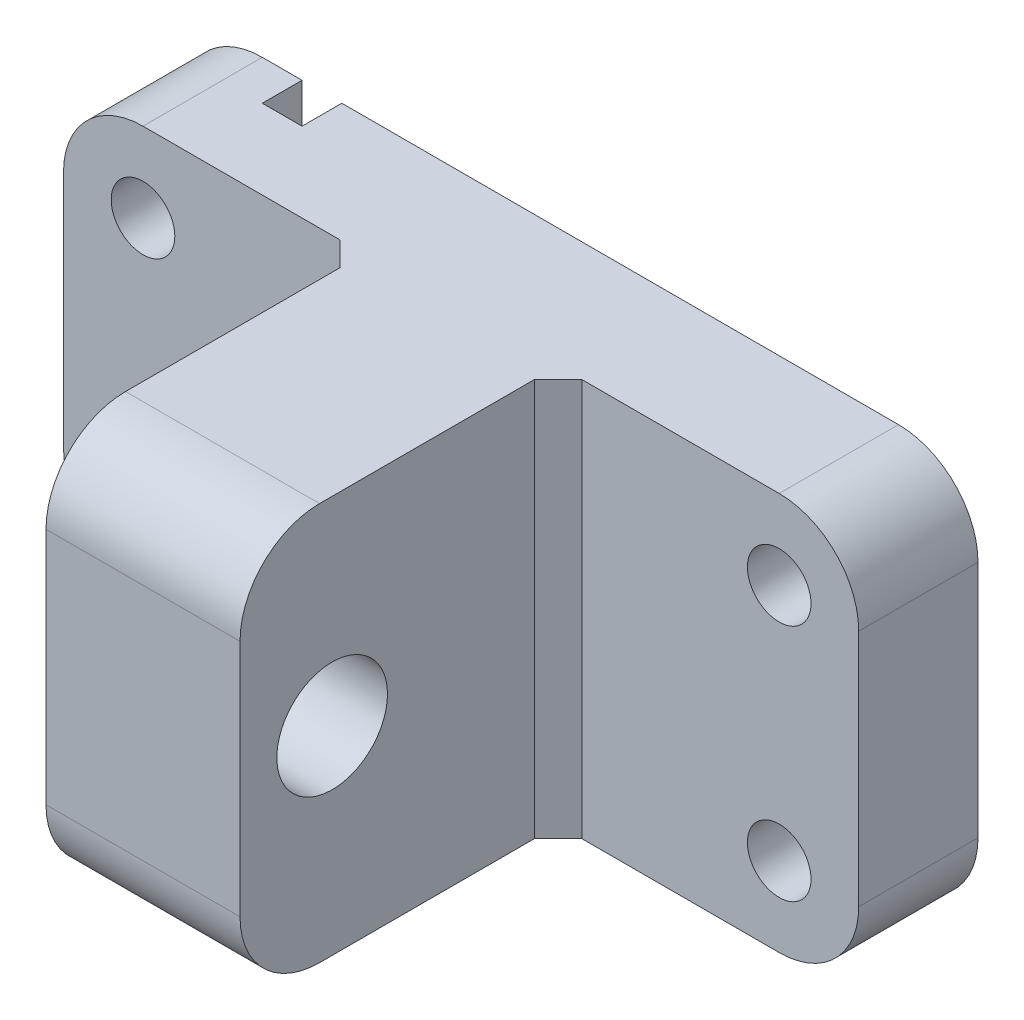
ISO-10303-21;
HEADER;
FILE_DESCRIPTION(('STEP AP214'),'2;1');
FILE_NAME('part.step','',(''),(''),'','','');
FILE_SCHEMA(('AUTOMOTIVE_DESIGN { 1 0 10303 214 1 1 1 1 }'));
ENDSEC;
DATA;
#1=APPLICATION_CONTEXT('core data for automotive mechanical design processes');
#2=APPLICATION_PROTOCOL_DEFINITION('international standard','automotive_design',2000,#1);
#3=PRODUCT_CONTEXT('',#1,'mechanical');
#4=PRODUCT('Part','Part','',(#3));
#5=PRODUCT_RELATED_PRODUCT_CATEGORY('part','',(#4));
#6=PRODUCT_DEFINITION_FORMATION('','',#4);
#7=PRODUCT_DEFINITION_CONTEXT('part definition',#1,'design');
#8=PRODUCT_DEFINITION('design','',#6,#7);
#9=PRODUCT_DEFINITION_SHAPE('','',#8);
#10=(LENGTH_UNIT() NAMED_UNIT(*) SI_UNIT(.MILLI.,.METRE.));
#11=(NAMED_UNIT(*) PLANE_ANGLE_UNIT() SI_UNIT($,.RADIAN.));
#12=(NAMED_UNIT(*) SI_UNIT($,.STERADIAN.) SOLID_ANGLE_UNIT());
#13=UNCERTAINTY_MEASURE_WITH_UNIT(LENGTH_MEASURE(1.E-05),#10,'distance_accuracy_value','');
#14=(GEOMETRIC_REPRESENTATION_CONTEXT(3) GLOBAL_UNCERTAINTY_ASSIGNED_CONTEXT((#13)) GLOBAL_UNIT_ASSIGNED_CONTEXT((#10,
#11,#12)) REPRESENTATION_CONTEXT('',''));
#15=CARTESIAN_POINT('',(0.,0.,0.));
#16=DIRECTION('',(0.,0.,1.));
#17=DIRECTION('',(1.,0.,0.));
#18=AXIS2_PLACEMENT_3D('',#15,#16,#17);
#19=CARTESIAN_POINT('',(90.,40.,0.));
#20=DIRECTION('',(0.,0.,1.));
#21=DIRECTION('',(1.,0.,0.));
#22=AXIS2_PLACEMENT_3D('',#19,#20,#21);
#23=PLANE('',#22);
#24=CARTESIAN_POINT('',(10.,40.,0.));
#25=DIRECTION('',(0.,0.,1.));
#26=DIRECTION('',(1.,0.,0.));
#27=AXIS2_PLACEMENT_3D('',#24,#25,#26);
#28=CIRCLE('',#27,4.);
#29=CARTESIAN_POINT('',(14.,40.,0.));
#30=VERTEX_POINT('',#29);
#31=EDGE_CURVE('E710',#30,#30,#28,.T.);
#32=ORIENTED_EDGE('',*,*,#31,.T.);
#33=EDGE_LOOP('',(#32));
#34=FACE_BOUND('',#33,.T.);
#35=CARTESIAN_POINT('',(10.,10.,0.));
#36=DIRECTION('',(0.,0.,1.));
#37=DIRECTION('',(1.,0.,0.));
#38=AXIS2_PLACEMENT_3D('',#35,#36,#37);
#39=CIRCLE('',#38,4.);
#40=CARTESIAN_POINT('',(14.,10.,0.));
#41=VERTEX_POINT('',#40);
#42=EDGE_CURVE('E712',#41,#41,#39,.T.);
#43=ORIENTED_EDGE('',*,*,#42,.T.);
#44=EDGE_LOOP('',(#43));
#45=FACE_BOUND('',#44,.T.);
#46=DIRECTION('',(-1.,0.,0.));
#47=VECTOR('',#46,1.);
#48=CARTESIAN_POINT('',(89.9999999999999,50.,0.));
#49=LINE('',#48,#47);
#50=CARTESIAN_POINT('',(15.,50.,0.));
#51=VERTEX_POINT('',#50);
#52=CARTESIAN_POINT('',(10.0000000000001,50.,0.));
#53=VERTEX_POINT('',#52);
#54=EDGE_CURVE('E287',#51,#53,#49,.T.);
#55=ORIENTED_EDGE('',*,*,#54,.F.);
#56=DIRECTION('',(0.,-1.,0.));
#57=VECTOR('',#56,1.);
#58=CARTESIAN_POINT('',(15.,50.,0.));
#59=LINE('',#58,#57);
#60=CARTESIAN_POINT('',(15.,0.,0.));
#61=VERTEX_POINT('',#60);
#62=EDGE_CURVE('E218',#51,#61,#59,.T.);
#63=ORIENTED_EDGE('',*,*,#62,.T.);
#64=DIRECTION('',(1.,0.,0.));
#65=VECTOR('',#64,1.);
#66=CARTESIAN_POINT('',(10.0000000000001,0.,0.));
#67=LINE('',#66,#65);
#68=CARTESIAN_POINT('',(10.0000000000001,0.,0.));
#69=VERTEX_POINT('',#68);
#70=EDGE_CURVE('E294',#69,#61,#67,.T.);
#71=ORIENTED_EDGE('',*,*,#70,.F.);
#72=CARTESIAN_POINT('',(10.,10.,0.));
#73=DIRECTION('',(0.,0.,1.));
#74=DIRECTION('',(-1.,0.,0.));
#75=AXIS2_PLACEMENT_3D('',#72,#73,#74);
#76=CIRCLE('',#75,10.);
#77=CARTESIAN_POINT('',(0.,10.,0.));
#78=VERTEX_POINT('',#77);
#79=EDGE_CURVE('E292',#78,#69,#76,.T.);
#80=ORIENTED_EDGE('',*,*,#79,.F.);
#81=DIRECTION('',(0.,-1.,0.));
#82=VECTOR('',#81,1.);
#83=CARTESIAN_POINT('',(0.,39.9999999999999,0.));
#84=LINE('',#83,#82);
#85=CARTESIAN_POINT('',(0.,39.9999999999999,0.));
#86=VERTEX_POINT('',#85);
#87=EDGE_CURVE('E288',#86,#78,#84,.T.);
#88=ORIENTED_EDGE('',*,*,#87,.F.);
#89=CARTESIAN_POINT('',(10.,40.,0.));
#90=DIRECTION('',(0.,0.,1.));
#91=DIRECTION('',(1.,0.,0.));
#92=AXIS2_PLACEMENT_3D('',#89,#90,#91);
#93=CIRCLE('',#92,10.);
#94=EDGE_CURVE('E290',#53,#86,#93,.T.);
#95=ORIENTED_EDGE('',*,*,#94,.F.);
#96=EDGE_LOOP('',(#55,#63,#71,#80,#88,#95));
#97=FACE_BOUND('',#96,.T.);
#98=ADVANCED_FACE('F50',(#34,#45,#97),#23,.F.);
#99=CARTESIAN_POINT('',(0.,10.,45.));
#100=DIRECTION('',(1.,0.,0.));
#101=DIRECTION('',(0.,0.,-1.));
#102=AXIS2_PLACEMENT_3D('',#99,#100,#101);
#103=CYLINDRICAL_SURFACE('',#102,10.);
#104=DIRECTION('',(1.,0.,0.));
#105=VECTOR('',#104,1.);
#106=CARTESIAN_POINT('',(0.,10.0000000000001,55.));
#107=LINE('',#106,#105);
#108=CARTESIAN_POINT('',(37.8,10.0000000000001,55.));
#109=VERTEX_POINT('',#108);
#110=CARTESIAN_POINT('',(62.2,9.99999999999993,55.));
#111=VERTEX_POINT('',#110);
#112=EDGE_CURVE('E267',#109,#111,#107,.T.);
#113=ORIENTED_EDGE('',*,*,#112,.F.);
#114=CARTESIAN_POINT('',(37.8,10.,45.));
#115=DIRECTION('',(-1.,0.,0.));
#116=DIRECTION('',(0.,0.,1.));
#117=AXIS2_PLACEMENT_3D('',#114,#115,#116);
#118=CIRCLE('',#117,10.);
#119=CARTESIAN_POINT('',(37.8,0.,45.0000000000001));
#120=VERTEX_POINT('',#119);
#121=EDGE_CURVE('E226',#120,#109,#118,.T.);
#122=ORIENTED_EDGE('',*,*,#121,.F.);
#123=DIRECTION('',(1.,0.,0.));
#124=VECTOR('',#123,1.);
#125=CARTESIAN_POINT('',(0.,0.,44.9999999999999));
#126=LINE('',#125,#124);
#127=CARTESIAN_POINT('',(62.2,0.,44.9999999999999));
#128=VERTEX_POINT('',#127);
#129=EDGE_CURVE('E265',#120,#128,#126,.T.);
#130=ORIENTED_EDGE('',*,*,#129,.T.);
#131=CARTESIAN_POINT('',(62.2,10.,45.));
#132=DIRECTION('',(1.,0.,0.));
#133=DIRECTION('',(0.,0.,-1.));
#134=AXIS2_PLACEMENT_3D('',#131,#132,#133);
#135=CIRCLE('',#134,10.);
#136=EDGE_CURVE('E252',#111,#128,#135,.T.);
#137=ORIENTED_EDGE('',*,*,#136,.F.);
#138=EDGE_LOOP('',(#113,#122,#130,#137));
#139=FACE_BOUND('',#138,.T.);
#140=ADVANCED_FACE('F348',(#139),#103,.T.);
#141=CARTESIAN_POINT('',(0.,39.9999999999999,55.));
#142=DIRECTION('',(0.,0.,1.));
#143=DIRECTION('',(1.,0.,0.));
#144=AXIS2_PLACEMENT_3D('',#141,#142,#143);
#145=PLANE('',#144);
#146=DIRECTION('',(1.,0.,0.));
#147=VECTOR('',#146,1.);
#148=CARTESIAN_POINT('',(0.,39.9999999999999,55.));
#149=LINE('',#148,#147);
#150=CARTESIAN_POINT('',(37.8,40.,55.));
#151=VERTEX_POINT('',#150);
#152=CARTESIAN_POINT('',(62.2,39.9999999999999,55.));
#153=VERTEX_POINT('',#152);
#154=EDGE_CURVE('E270',#151,#153,#149,.T.);
#155=ORIENTED_EDGE('',*,*,#154,.F.);
#156=DIRECTION('',(0.,1.,0.));
#157=VECTOR('',#156,1.);
#158=CARTESIAN_POINT('',(37.8,40.,55.));
#159=LINE('',#158,#157);
#160=EDGE_CURVE('E229',#109,#151,#159,.T.);
#161=ORIENTED_EDGE('',*,*,#160,.F.);
#162=ORIENTED_EDGE('',*,*,#112,.T.);
#163=DIRECTION('',(0.,-1.,0.));
#164=VECTOR('',#163,1.);
#165=CARTESIAN_POINT('',(62.2,39.9999999999999,55.));
#166=LINE('',#165,#164);
#167=EDGE_CURVE('E247',#153,#111,#166,.T.);
#168=ORIENTED_EDGE('',*,*,#167,.F.);
#169=EDGE_LOOP('',(#155,#161,#162,#168));
#170=FACE_BOUND('',#169,.T.);
#171=ADVANCED_FACE('F356',(#170),#145,.T.);
#172=CARTESIAN_POINT('',(0.,40.,45.));
#173=DIRECTION('',(1.,0.,0.));
#174=DIRECTION('',(0.,0.,-1.));
#175=AXIS2_PLACEMENT_3D('',#172,#173,#174);
#176=CYLINDRICAL_SURFACE('',#175,10.);
#177=DIRECTION('',(1.,0.,0.));
#178=VECTOR('',#177,1.);
#179=CARTESIAN_POINT('',(0.,50.,44.9999999999999));
#180=LINE('',#179,#178);
#181=CARTESIAN_POINT('',(37.8,50.,45.));
#182=VERTEX_POINT('',#181);
#183=CARTESIAN_POINT('',(62.2,50.,44.9999999999999));
#184=VERTEX_POINT('',#183);
#185=EDGE_CURVE('E262',#182,#184,#180,.T.);
#186=ORIENTED_EDGE('',*,*,#185,.F.);
#187=CARTESIAN_POINT('',(37.8,40.,45.));
#188=DIRECTION('',(-1.,0.,0.));
#189=DIRECTION('',(0.,0.,1.));
#190=AXIS2_PLACEMENT_3D('',#187,#188,#189);
#191=CIRCLE('',#190,9.99999999999999);
#192=EDGE_CURVE('E235',#151,#182,#191,.T.);
#193=ORIENTED_EDGE('',*,*,#192,.F.);
#194=ORIENTED_EDGE('',*,*,#154,.T.);
#195=CARTESIAN_POINT('',(62.2,40.,45.));
#196=DIRECTION('',(1.,0.,0.));
#197=DIRECTION('',(0.,0.,-1.));
#198=AXIS2_PLACEMENT_3D('',#195,#196,#197);
#199=CIRCLE('',#198,9.99999999999999);
#200=EDGE_CURVE('E244',#184,#153,#199,.T.);
#201=ORIENTED_EDGE('',*,*,#200,.F.);
#202=EDGE_LOOP('',(#186,#193,#194,#201));
#203=FACE_BOUND('',#202,.T.);
#204=ADVANCED_FACE('F361',(#203),#176,.T.);
#205=CARTESIAN_POINT('',(90.,40.,15.));
#206=DIRECTION('',(0.,0.,-1.));
#207=DIRECTION('',(-1.,0.,0.));
#208=AXIS2_PLACEMENT_3D('',#205,#206,#207);
#209=CYLINDRICAL_SURFACE('',#208,9.99999999999999);
#210=CARTESIAN_POINT('',(90.,40.,0.));
#211=DIRECTION('',(0.,0.,1.));
#212=DIRECTION('',(1.,0.,0.));
#213=AXIS2_PLACEMENT_3D('',#210,#211,#212);
#214=CIRCLE('',#213,9.99999999999999);
#215=CARTESIAN_POINT('',(100.,39.9999999999999,0.));
#216=VERTEX_POINT('',#215);
#217=CARTESIAN_POINT('',(89.9999999999999,50.,0.));
#218=VERTEX_POINT('',#217);
#219=EDGE_CURVE('E263',#216,#218,#214,.T.);
#220=ORIENTED_EDGE('',*,*,#219,.T.);
#221=DIRECTION('',(0.,0.,-1.));
#222=VECTOR('',#221,1.);
#223=CARTESIAN_POINT('',(89.9999999999999,50.,15.));
#224=LINE('',#223,#222);
#225=CARTESIAN_POINT('',(90.,50.,15.));
#226=VERTEX_POINT('',#225);
#227=EDGE_CURVE('E322',#226,#218,#224,.T.);
#228=ORIENTED_EDGE('',*,*,#227,.F.);
#229=CARTESIAN_POINT('',(90.,40.,15.));
#230=DIRECTION('',(0.,0.,1.));
#231=DIRECTION('',(1.,0.,0.));
#232=AXIS2_PLACEMENT_3D('',#229,#230,#231);
#233=CIRCLE('',#232,9.99999999999999);
#234=CARTESIAN_POINT('',(100.,40.,15.));
#235=VERTEX_POINT('',#234);
#236=EDGE_CURVE('E275',#235,#226,#233,.T.);
#237=ORIENTED_EDGE('',*,*,#236,.F.);
#238=DIRECTION('',(0.,0.,-1.));
#239=VECTOR('',#238,1.);
#240=CARTESIAN_POINT('',(100.,39.9999999999999,15.));
#241=LINE('',#240,#239);
#242=EDGE_CURVE('E285',#235,#216,#241,.T.);
#243=ORIENTED_EDGE('',*,*,#242,.T.);
#244=EDGE_LOOP('',(#220,#228,#237,#243));
#245=FACE_BOUND('',#244,.T.);
#246=ADVANCED_FACE('F425',(#245),#209,.T.);
#247=CARTESIAN_POINT('',(89.9999999999999,50.,15.));
#248=DIRECTION('',(0.,-1.,0.));
#249=DIRECTION('',(0.,0.,-1.));
#250=AXIS2_PLACEMENT_3D('',#247,#248,#249);
#251=PLANE('',#250);
#252=DIRECTION('',(-1.,0.,0.));
#253=VECTOR('',#252,1.);
#254=CARTESIAN_POINT('',(15.,50.,5.));
#255=LINE('',#254,#253);
#256=CARTESIAN_POINT('',(20.,50.,5.));
#257=VERTEX_POINT('',#256);
#258=CARTESIAN_POINT('',(15.,50.,5.));
#259=VERTEX_POINT('',#258);
#260=EDGE_CURVE('E199',#257,#259,#255,.T.);
#261=ORIENTED_EDGE('',*,*,#260,.T.);
#262=DIRECTION('',(0.,0.,-1.));
#263=VECTOR('',#262,1.);
#264=CARTESIAN_POINT('',(15.,50.,0.));
#265=LINE('',#264,#263);
#266=EDGE_CURVE('E204',#259,#51,#265,.T.);
#267=ORIENTED_EDGE('',*,*,#266,.T.);
#268=ORIENTED_EDGE('',*,*,#54,.T.);
#269=DIRECTION('',(0.,0.,-1.));
#270=VECTOR('',#269,1.);
#271=CARTESIAN_POINT('',(10.0000000000001,50.,15.));
#272=LINE('',#271,#270);
#273=CARTESIAN_POINT('',(10.,50.,15.));
#274=VERTEX_POINT('',#273);
#275=EDGE_CURVE('E319',#274,#53,#272,.T.);
#276=ORIENTED_EDGE('',*,*,#275,.F.);
#277=DIRECTION('',(-1.,0.,0.));
#278=VECTOR('',#277,1.);
#279=CARTESIAN_POINT('',(37.8,50.,15.));
#280=LINE('',#279,#278);
#281=CARTESIAN_POINT('',(34.8,50.,15.));
#282=VERTEX_POINT('',#281);
#283=EDGE_CURVE('E237',#282,#274,#280,.T.);
#284=ORIENTED_EDGE('',*,*,#283,.F.);
#285=DIRECTION('',(0.707106781186544,0.,0.707106781186551));
#286=VECTOR('',#285,1.);
#287=CARTESIAN_POINT('',(62.3999999999997,50.,42.6));
#288=LINE('',#287,#286);
#289=CARTESIAN_POINT('',(37.8,50.,18.));
#290=VERTEX_POINT('',#289);
#291=EDGE_CURVE('E11',#282,#290,#288,.T.);
#292=ORIENTED_EDGE('',*,*,#291,.T.);
#293=DIRECTION('',(0.,0.,-1.));
#294=VECTOR('',#293,1.);
#295=CARTESIAN_POINT('',(37.8,50.,15.));
#296=LINE('',#295,#294);
#297=EDGE_CURVE('E234',#182,#290,#296,.T.);
#298=ORIENTED_EDGE('',*,*,#297,.F.);
#299=ORIENTED_EDGE('',*,*,#185,.T.);
#300=DIRECTION('',(0.,0.,1.));
#301=VECTOR('',#300,1.);
#302=CARTESIAN_POINT('',(62.2,50.,15.));
#303=LINE('',#302,#301);
#304=CARTESIAN_POINT('',(62.2,50.,18.));
#305=VERTEX_POINT('',#304);
#306=EDGE_CURVE('E243',#305,#184,#303,.T.);
#307=ORIENTED_EDGE('',*,*,#306,.F.);
#308=DIRECTION('',(0.707106781186544,0.,-0.707106781186551));
#309=VECTOR('',#308,1.);
#310=CARTESIAN_POINT('',(77.5999999999999,50.,2.60000000000003));
#311=LINE('',#310,#309);
#312=CARTESIAN_POINT('',(65.2,50.,15.));
#313=VERTEX_POINT('',#312);
#314=EDGE_CURVE('E328',#305,#313,#311,.T.);
#315=ORIENTED_EDGE('',*,*,#314,.T.);
#316=DIRECTION('',(1.,0.,0.));
#317=VECTOR('',#316,1.);
#318=CARTESIAN_POINT('',(62.2,50.,15.));
#319=LINE('',#318,#317);
#320=EDGE_CURVE('E260',#313,#226,#319,.T.);
#321=ORIENTED_EDGE('',*,*,#320,.T.);
#322=ORIENTED_EDGE('',*,*,#227,.T.);
#323=CARTESIAN_POINT('',(20.,50.,0.));
#324=VERTEX_POINT('',#323);
#325=EDGE_CURVE('E210',#218,#324,#49,.T.);
#326=ORIENTED_EDGE('',*,*,#325,.T.);
#327=DIRECTION('',(0.,0.,1.));
#328=VECTOR('',#327,1.);
#329=CARTESIAN_POINT('',(20.,50.,5.));
#330=LINE('',#329,#328);
#331=EDGE_CURVE('E187',#324,#257,#330,.T.);
#332=ORIENTED_EDGE('',*,*,#331,.T.);
#333=EDGE_LOOP('',(#261,#267,#268,#276,#284,#292,#298,#299,#307,#315,#321,#322,#326,#332));
#334=FACE_BOUND('',#333,.T.);
#335=ADVANCED_FACE('F203',(#334),#251,.F.);
#336=CARTESIAN_POINT('',(10.,40.,15.));
#337=DIRECTION('',(0.,0.,-1.));
#338=DIRECTION('',(-1.,0.,0.));
#339=AXIS2_PLACEMENT_3D('',#336,#337,#338);
#340=CYLINDRICAL_SURFACE('',#339,10.);
#341=ORIENTED_EDGE('',*,*,#94,.T.);
#342=DIRECTION('',(0.,0.,-1.));
#343=VECTOR('',#342,1.);
#344=CARTESIAN_POINT('',(0.,39.9999999999999,15.));
#345=LINE('',#344,#343);
#346=CARTESIAN_POINT('',(0.,40.,15.));
#347=VERTEX_POINT('',#346);
#348=EDGE_CURVE('E314',#347,#86,#345,.T.);
#349=ORIENTED_EDGE('',*,*,#348,.F.);
#350=CARTESIAN_POINT('',(10.,40.,15.));
#351=DIRECTION('',(0.,0.,1.));
#352=DIRECTION('',(1.,0.,0.));
#353=AXIS2_PLACEMENT_3D('',#350,#351,#352);
#354=CIRCLE('',#353,10.);
#355=EDGE_CURVE('E273',#274,#347,#354,.T.);
#356=ORIENTED_EDGE('',*,*,#355,.F.);
#357=ORIENTED_EDGE('',*,*,#275,.T.);
#358=EDGE_LOOP('',(#341,#349,#356,#357));
#359=FACE_BOUND('',#358,.T.);
#360=ADVANCED_FACE('F433',(#359),#340,.T.);
#361=CARTESIAN_POINT('',(0.,39.9999999999999,15.));
#362=DIRECTION('',(1.,0.,0.));
#363=DIRECTION('',(0.,0.,-1.));
#364=AXIS2_PLACEMENT_3D('',#361,#362,#363);
#365=PLANE('',#364);
#366=DIRECTION('',(0.,0.,-1.));
#367=VECTOR('',#366,1.);
#368=CARTESIAN_POINT('',(0.,10.,15.));
#369=LINE('',#368,#367);
#370=CARTESIAN_POINT('',(0.,9.99999999999999,15.));
#371=VERTEX_POINT('',#370);
#372=EDGE_CURVE('E315',#371,#78,#369,.T.);
#373=ORIENTED_EDGE('',*,*,#372,.F.);
#374=DIRECTION('',(0.,-1.,0.));
#375=VECTOR('',#374,1.);
#376=CARTESIAN_POINT('',(0.,50.,15.));
#377=LINE('',#376,#375);
#378=EDGE_CURVE('E225',#347,#371,#377,.T.);
#379=ORIENTED_EDGE('',*,*,#378,.F.);
#380=ORIENTED_EDGE('',*,*,#348,.T.);
#381=ORIENTED_EDGE('',*,*,#87,.T.);
#382=EDGE_LOOP('',(#373,#379,#380,#381));
#383=FACE_BOUND('',#382,.T.);
#384=ADVANCED_FACE('F443',(#383),#365,.F.);
#385=CARTESIAN_POINT('',(10.,10.,15.));
#386=DIRECTION('',(0.,0.,-1.));
#387=DIRECTION('',(-1.,0.,0.));
#388=AXIS2_PLACEMENT_3D('',#385,#386,#387);
#389=CYLINDRICAL_SURFACE('',#388,10.);
#390=ORIENTED_EDGE('',*,*,#79,.T.);
#391=DIRECTION('',(0.,0.,-1.));
#392=VECTOR('',#391,1.);
#393=CARTESIAN_POINT('',(10.0000000000001,0.,15.));
#394=LINE('',#393,#392);
#395=CARTESIAN_POINT('',(10.,0.,15.));
#396=VERTEX_POINT('',#395);
#397=EDGE_CURVE('E307',#396,#69,#394,.T.);
#398=ORIENTED_EDGE('',*,*,#397,.F.);
#399=CARTESIAN_POINT('',(10.,10.,15.));
#400=DIRECTION('',(0.,0.,1.));
#401=DIRECTION('',(-1.,0.,0.));
#402=AXIS2_PLACEMENT_3D('',#399,#400,#401);
#403=CIRCLE('',#402,10.);
#404=EDGE_CURVE('E279',#371,#396,#403,.T.);
#405=ORIENTED_EDGE('',*,*,#404,.F.);
#406=ORIENTED_EDGE('',*,*,#372,.T.);
#407=EDGE_LOOP('',(#390,#398,#405,#406));
#408=FACE_BOUND('',#407,.T.);
#409=ADVANCED_FACE('F449',(#408),#389,.T.);
#410=CARTESIAN_POINT('',(10.0000000000001,0.,15.));
#411=DIRECTION('',(0.,1.,0.));
#412=DIRECTION('',(0.,0.,1.));
#413=AXIS2_PLACEMENT_3D('',#410,#411,#412);
#414=PLANE('',#413);
#415=ORIENTED_EDGE('',*,*,#70,.T.);
#416=DIRECTION('',(0.,0.,-1.));
#417=VECTOR('',#416,1.);
#418=CARTESIAN_POINT('',(15.,0.,0.));
#419=LINE('',#418,#417);
#420=CARTESIAN_POINT('',(15.,0.,5.));
#421=VERTEX_POINT('',#420);
#422=EDGE_CURVE('E206',#421,#61,#419,.T.);
#423=ORIENTED_EDGE('',*,*,#422,.F.);
#424=DIRECTION('',(-1.,0.,0.));
#425=VECTOR('',#424,1.);
#426=CARTESIAN_POINT('',(15.,0.,5.));
#427=LINE('',#426,#425);
#428=CARTESIAN_POINT('',(20.,0.,5.));
#429=VERTEX_POINT('',#428);
#430=EDGE_CURVE('E208',#429,#421,#427,.T.);
#431=ORIENTED_EDGE('',*,*,#430,.F.);
#432=DIRECTION('',(0.,0.,1.));
#433=VECTOR('',#432,1.);
#434=CARTESIAN_POINT('',(20.,0.,5.));
#435=LINE('',#434,#433);
#436=CARTESIAN_POINT('',(20.,0.,0.));
#437=VERTEX_POINT('',#436);
#438=EDGE_CURVE('E186',#437,#429,#435,.T.);
#439=ORIENTED_EDGE('',*,*,#438,.F.);
#440=CARTESIAN_POINT('',(89.9999999999999,0.,0.));
#441=VERTEX_POINT('',#440);
#442=EDGE_CURVE('E295',#437,#441,#67,.T.);
#443=ORIENTED_EDGE('',*,*,#442,.T.);
#444=DIRECTION('',(0.,0.,-1.));
#445=VECTOR('',#444,1.);
#446=CARTESIAN_POINT('',(89.9999999999999,0.,15.));
#447=LINE('',#446,#445);
#448=CARTESIAN_POINT('',(90.,0.,15.));
#449=VERTEX_POINT('',#448);
#450=EDGE_CURVE('E306',#449,#441,#447,.T.);
#451=ORIENTED_EDGE('',*,*,#450,.F.);
#452=DIRECTION('',(1.,0.,0.));
#453=VECTOR('',#452,1.);
#454=CARTESIAN_POINT('',(62.2,0.,15.));
#455=LINE('',#454,#453);
#456=CARTESIAN_POINT('',(65.2,0.,15.));
#457=VERTEX_POINT('',#456);
#458=EDGE_CURVE('E256',#457,#449,#455,.T.);
#459=ORIENTED_EDGE('',*,*,#458,.F.);
#460=DIRECTION('',(-0.707106781186544,0.,0.707106781186551));
#461=VECTOR('',#460,1.);
#462=CARTESIAN_POINT('',(37.6000000000003,0.,42.6));
#463=LINE('',#462,#461);
#464=CARTESIAN_POINT('',(62.2,0.,18.));
#465=VERTEX_POINT('',#464);
#466=EDGE_CURVE('E334',#457,#465,#463,.T.);
#467=ORIENTED_EDGE('',*,*,#466,.T.);
#468=DIRECTION('',(0.,0.,-1.));
#469=VECTOR('',#468,1.);
#470=CARTESIAN_POINT('',(62.2,0.,44.9999999999999));
#471=LINE('',#470,#469);
#472=EDGE_CURVE('E251',#128,#465,#471,.T.);
#473=ORIENTED_EDGE('',*,*,#472,.F.);
#474=ORIENTED_EDGE('',*,*,#129,.F.);
#475=DIRECTION('',(0.,0.,1.));
#476=VECTOR('',#475,1.);
#477=CARTESIAN_POINT('',(37.8,0.,15.));
#478=LINE('',#477,#476);
#479=CARTESIAN_POINT('',(37.8,0.,18.));
#480=VERTEX_POINT('',#479);
#481=EDGE_CURVE('E228',#480,#120,#478,.T.);
#482=ORIENTED_EDGE('',*,*,#481,.F.);
#483=DIRECTION('',(-0.707106781186544,0.,-0.707106781186551));
#484=VECTOR('',#483,1.);
#485=CARTESIAN_POINT('',(22.4000000000002,0.,2.60000000000003));
#486=LINE('',#485,#484);
#487=CARTESIAN_POINT('',(34.8,0.,15.));
#488=VERTEX_POINT('',#487);
#489=EDGE_CURVE('E57',#480,#488,#486,.T.);
#490=ORIENTED_EDGE('',*,*,#489,.T.);
#491=DIRECTION('',(-1.,0.,0.));
#492=VECTOR('',#491,1.);
#493=CARTESIAN_POINT('',(37.8,0.,15.));
#494=LINE('',#493,#492);
#495=EDGE_CURVE('E240',#488,#396,#494,.T.);
#496=ORIENTED_EDGE('',*,*,#495,.T.);
#497=ORIENTED_EDGE('',*,*,#397,.T.);
#498=EDGE_LOOP('',(#415,#423,#431,#439,#443,#451,#459,#467,#473,#474,#482,#490,#496,#497));
#499=FACE_BOUND('',#498,.T.);
#500=ADVANCED_FACE('F343',(#499),#414,.F.);
#501=CARTESIAN_POINT('',(90.,10.,15.));
#502=DIRECTION('',(0.,0.,-1.));
#503=DIRECTION('',(-1.,0.,0.));
#504=AXIS2_PLACEMENT_3D('',#501,#502,#503);
#505=CYLINDRICAL_SURFACE('',#504,10.);
#506=CARTESIAN_POINT('',(90.,10.,0.));
#507=DIRECTION('',(0.,0.,1.));
#508=DIRECTION('',(1.,0.,0.));
#509=AXIS2_PLACEMENT_3D('',#506,#507,#508);
#510=CIRCLE('',#509,10.);
#511=CARTESIAN_POINT('',(100.,10.0000000000001,0.));
#512=VERTEX_POINT('',#511);
#513=EDGE_CURVE('E296',#441,#512,#510,.T.);
#514=ORIENTED_EDGE('',*,*,#513,.T.);
#515=DIRECTION('',(0.,0.,-1.));
#516=VECTOR('',#515,1.);
#517=CARTESIAN_POINT('',(100.,10.0000000000001,15.));
#518=LINE('',#517,#516);
#519=CARTESIAN_POINT('',(100.,9.99999999999999,15.));
#520=VERTEX_POINT('',#519);
#521=EDGE_CURVE('E303',#520,#512,#518,.T.);
#522=ORIENTED_EDGE('',*,*,#521,.F.);
#523=CARTESIAN_POINT('',(90.,10.,15.));
#524=DIRECTION('',(0.,0.,1.));
#525=DIRECTION('',(1.,0.,0.));
#526=AXIS2_PLACEMENT_3D('',#523,#524,#525);
#527=CIRCLE('',#526,10.);
#528=EDGE_CURVE('E282',#449,#520,#527,.T.);
#529=ORIENTED_EDGE('',*,*,#528,.F.);
#530=ORIENTED_EDGE('',*,*,#450,.T.);
#531=EDGE_LOOP('',(#514,#522,#529,#530));
#532=FACE_BOUND('',#531,.T.);
#533=ADVANCED_FACE('F400',(#532),#505,.T.);
#534=CARTESIAN_POINT('',(100.,10.0000000000001,15.));
#535=DIRECTION('',(-1.,0.,0.));
#536=DIRECTION('',(0.,0.,1.));
#537=AXIS2_PLACEMENT_3D('',#534,#535,#536);
#538=PLANE('',#537);
#539=ORIENTED_EDGE('',*,*,#242,.F.);
#540=DIRECTION('',(0.,1.,0.));
#541=VECTOR('',#540,1.);
#542=CARTESIAN_POINT('',(100.,39.9999999999999,15.));
#543=LINE('',#542,#541);
#544=EDGE_CURVE('E241',#520,#235,#543,.T.);
#545=ORIENTED_EDGE('',*,*,#544,.F.);
#546=ORIENTED_EDGE('',*,*,#521,.T.);
#547=DIRECTION('',(0.,1.,0.));
#548=VECTOR('',#547,1.);
#549=CARTESIAN_POINT('',(100.,10.0000000000001,0.));
#550=LINE('',#549,#548);
#551=EDGE_CURVE('E277',#512,#216,#550,.T.);
#552=ORIENTED_EDGE('',*,*,#551,.T.);
#553=EDGE_LOOP('',(#539,#545,#546,#552));
#554=FACE_BOUND('',#553,.T.);
#555=ADVANCED_FACE('F386',(#554),#538,.F.);
#556=CARTESIAN_POINT('',(90.,10.,0.));
#557=DIRECTION('',(0.,0.,1.));
#558=DIRECTION('',(1.,0.,0.));
#559=AXIS2_PLACEMENT_3D('',#556,#557,#558);
#560=CIRCLE('',#559,4.00000000000001);
#561=CARTESIAN_POINT('',(94.,10.,0.));
#562=VERTEX_POINT('',#561);
#563=EDGE_CURVE('E401',#562,#562,#560,.T.);
#564=ORIENTED_EDGE('',*,*,#563,.T.);
#565=EDGE_LOOP('',(#564));
#566=FACE_BOUND('',#565,.T.);
#567=CARTESIAN_POINT('',(90.,40.,0.));
#568=DIRECTION('',(0.,0.,1.));
#569=DIRECTION('',(1.,0.,0.));
#570=AXIS2_PLACEMENT_3D('',#567,#568,#569);
#571=CIRCLE('',#570,3.99999999999999);
#572=CARTESIAN_POINT('',(94.,40.,0.));
#573=VERTEX_POINT('',#572);
#574=EDGE_CURVE('E410',#573,#573,#571,.T.);
#575=ORIENTED_EDGE('',*,*,#574,.T.);
#576=EDGE_LOOP('',(#575));
#577=FACE_BOUND('',#576,.T.);
#578=ORIENTED_EDGE('',*,*,#442,.F.);
#579=DIRECTION('',(0.,-1.,0.));
#580=VECTOR('',#579,1.);
#581=CARTESIAN_POINT('',(20.,50.,0.));
#582=LINE('',#581,#580);
#583=EDGE_CURVE('E191',#324,#437,#582,.T.);
#584=ORIENTED_EDGE('',*,*,#583,.F.);
#585=ORIENTED_EDGE('',*,*,#325,.F.);
#586=ORIENTED_EDGE('',*,*,#219,.F.);
#587=ORIENTED_EDGE('',*,*,#551,.F.);
#588=ORIENTED_EDGE('',*,*,#513,.F.);
#589=EDGE_LOOP('',(#578,#584,#585,#586,#587,#588));
#590=FACE_BOUND('',#589,.T.);
#591=ADVANCED_FACE('F380',(#566,#577,#590),#23,.F.);
#592=CARTESIAN_POINT('',(62.2,39.9999999999999,15.));
#593=DIRECTION('',(0.,0.,-1.));
#594=DIRECTION('',(-1.,0.,0.));
#595=AXIS2_PLACEMENT_3D('',#592,#593,#594);
#596=PLANE('',#595);
#597=CARTESIAN_POINT('',(90.,10.,15.));
#598=DIRECTION('',(0.,0.,1.));
#599=DIRECTION('',(1.,0.,0.));
#600=AXIS2_PLACEMENT_3D('',#597,#598,#599);
#601=CIRCLE('',#600,4.00000000000001);
#602=CARTESIAN_POINT('',(94.,10.,15.));
#603=VERTEX_POINT('',#602);
#604=EDGE_CURVE('E719',#603,#603,#601,.T.);
#605=ORIENTED_EDGE('',*,*,#604,.F.);
#606=EDGE_LOOP('',(#605));
#607=FACE_BOUND('',#606,.T.);
#608=CARTESIAN_POINT('',(90.,40.,15.));
#609=DIRECTION('',(0.,0.,1.));
#610=DIRECTION('',(1.,0.,0.));
#611=AXIS2_PLACEMENT_3D('',#608,#609,#610);
#612=CIRCLE('',#611,3.99999999999999);
#613=CARTESIAN_POINT('',(94.,40.,15.));
#614=VERTEX_POINT('',#613);
#615=EDGE_CURVE('E711',#614,#614,#612,.T.);
#616=ORIENTED_EDGE('',*,*,#615,.F.);
#617=EDGE_LOOP('',(#616));
#618=FACE_BOUND('',#617,.T.);
#619=ORIENTED_EDGE('',*,*,#320,.F.);
#620=DIRECTION('',(0.,-1.,0.));
#621=VECTOR('',#620,1.);
#622=CARTESIAN_POINT('',(65.2,39.9999999999999,15.));
#623=LINE('',#622,#621);
#624=EDGE_CURVE('E330',#313,#457,#623,.T.);
#625=ORIENTED_EDGE('',*,*,#624,.T.);
#626=ORIENTED_EDGE('',*,*,#458,.T.);
#627=ORIENTED_EDGE('',*,*,#528,.T.);
#628=ORIENTED_EDGE('',*,*,#544,.T.);
#629=ORIENTED_EDGE('',*,*,#236,.T.);
#630=EDGE_LOOP('',(#619,#625,#626,#627,#628,#629));
#631=FACE_BOUND('',#630,.T.);
#632=ADVANCED_FACE('F389',(#607,#618,#631),#596,.F.);
#633=CARTESIAN_POINT('',(62.2,40.,45.));
#634=DIRECTION('',(1.,0.,0.));
#635=DIRECTION('',(0.,0.,-1.));
#636=AXIS2_PLACEMENT_3D('',#633,#634,#635);
#637=PLANE('',#636);
#638=CARTESIAN_POINT('',(62.2,25.,43.4159709081373));
#639=DIRECTION('',(1.,0.,0.));
#640=DIRECTION('',(0.,0.,-1.));
#641=AXIS2_PLACEMENT_3D('',#638,#639,#640);
#642=CIRCLE('',#641,6.95795029846374);
#643=CARTESIAN_POINT('',(62.2,25.,36.4580206096735));
#644=VERTEX_POINT('',#643);
#645=EDGE_CURVE('E214',#644,#644,#642,.T.);
#646=ORIENTED_EDGE('',*,*,#645,.F.);
#647=EDGE_LOOP('',(#646));
#648=FACE_BOUND('',#647,.T.);
#649=ORIENTED_EDGE('',*,*,#472,.T.);
#650=DIRECTION('',(0.,1.,0.));
#651=VECTOR('',#650,1.);
#652=CARTESIAN_POINT('',(62.2,40.,18.));
#653=LINE('',#652,#651);
#654=EDGE_CURVE('E324',#465,#305,#653,.T.);
#655=ORIENTED_EDGE('',*,*,#654,.T.);
#656=ORIENTED_EDGE('',*,*,#306,.T.);
#657=ORIENTED_EDGE('',*,*,#200,.T.);
#658=ORIENTED_EDGE('',*,*,#167,.T.);
#659=ORIENTED_EDGE('',*,*,#136,.T.);
#660=EDGE_LOOP('',(#649,#655,#656,#657,#658,#659));
#661=FACE_BOUND('',#660,.T.);
#662=ADVANCED_FACE('F354',(#648,#661),#637,.T.);
#663=CARTESIAN_POINT('',(37.8,50.,15.));
#664=DIRECTION('',(0.,0.,-1.));
#665=DIRECTION('',(-1.,0.,0.));
#666=AXIS2_PLACEMENT_3D('',#663,#664,#665);
#667=PLANE('',#666);
#668=CARTESIAN_POINT('',(10.,40.,15.));
#669=DIRECTION('',(0.,0.,1.));
#670=DIRECTION('',(1.,0.,0.));
#671=AXIS2_PLACEMENT_3D('',#668,#669,#670);
#672=CIRCLE('',#671,4.);
#673=CARTESIAN_POINT('',(14.,40.,15.));
#674=VERTEX_POINT('',#673);
#675=EDGE_CURVE('E720',#674,#674,#672,.T.);
#676=ORIENTED_EDGE('',*,*,#675,.F.);
#677=EDGE_LOOP('',(#676));
#678=FACE_BOUND('',#677,.T.);
#679=CARTESIAN_POINT('',(10.,10.,15.));
#680=DIRECTION('',(0.,0.,1.));
#681=DIRECTION('',(1.,0.,0.));
#682=AXIS2_PLACEMENT_3D('',#679,#680,#681);
#683=CIRCLE('',#682,4.);
#684=CARTESIAN_POINT('',(14.,10.,15.));
#685=VERTEX_POINT('',#684);
#686=EDGE_CURVE('E722',#685,#685,#683,.T.);
#687=ORIENTED_EDGE('',*,*,#686,.F.);
#688=EDGE_LOOP('',(#687));
#689=FACE_BOUND('',#688,.T.);
#690=ORIENTED_EDGE('',*,*,#495,.F.);
#691=DIRECTION('',(0.,1.,0.));
#692=VECTOR('',#691,1.);
#693=CARTESIAN_POINT('',(34.8,50.,15.));
#694=LINE('',#693,#692);
#695=EDGE_CURVE('E64',#488,#282,#694,.T.);
#696=ORIENTED_EDGE('',*,*,#695,.T.);
#697=ORIENTED_EDGE('',*,*,#283,.T.);
#698=ORIENTED_EDGE('',*,*,#355,.T.);
#699=ORIENTED_EDGE('',*,*,#378,.T.);
#700=ORIENTED_EDGE('',*,*,#404,.T.);
#701=EDGE_LOOP('',(#690,#696,#697,#698,#699,#700));
#702=FACE_BOUND('',#701,.T.);
#703=ADVANCED_FACE('F610',(#678,#689,#702),#667,.F.);
#704=CARTESIAN_POINT('',(37.8,10.,45.));
#705=DIRECTION('',(-1.,0.,0.));
#706=DIRECTION('',(0.,0.,1.));
#707=AXIS2_PLACEMENT_3D('',#704,#705,#706);
#708=PLANE('',#707);
#709=CARTESIAN_POINT('',(37.8,25.,43.4159709081373));
#710=DIRECTION('',(-1.,0.,0.));
#711=DIRECTION('',(0.,0.,1.));
#712=AXIS2_PLACEMENT_3D('',#709,#710,#711);
#713=CIRCLE('',#712,6.95795029846374);
#714=CARTESIAN_POINT('',(37.8,25.,50.373921206601));
#715=VERTEX_POINT('',#714);
#716=EDGE_CURVE('E220',#715,#715,#713,.T.);
#717=ORIENTED_EDGE('',*,*,#716,.F.);
#718=EDGE_LOOP('',(#717));
#719=FACE_BOUND('',#718,.T.);
#720=ORIENTED_EDGE('',*,*,#297,.T.);
#721=DIRECTION('',(0.,-1.,0.));
#722=VECTOR('',#721,1.);
#723=CARTESIAN_POINT('',(37.8,10.,18.));
#724=LINE('',#723,#722);
#725=EDGE_CURVE('E331',#290,#480,#724,.T.);
#726=ORIENTED_EDGE('',*,*,#725,.T.);
#727=ORIENTED_EDGE('',*,*,#481,.T.);
#728=ORIENTED_EDGE('',*,*,#121,.T.);
#729=ORIENTED_EDGE('',*,*,#160,.T.);
#730=ORIENTED_EDGE('',*,*,#192,.T.);
#731=EDGE_LOOP('',(#720,#726,#727,#728,#729,#730));
#732=FACE_BOUND('',#731,.T.);
#733=ADVANCED_FACE('F339',(#719,#732),#708,.T.);
#734=CARTESIAN_POINT('',(15.,50.,0.));
#735=DIRECTION('',(-1.,0.,0.));
#736=DIRECTION('',(0.,0.,1.));
#737=AXIS2_PLACEMENT_3D('',#734,#735,#736);
#738=PLANE('',#737);
#739=ORIENTED_EDGE('',*,*,#422,.T.);
#740=ORIENTED_EDGE('',*,*,#62,.F.);
#741=ORIENTED_EDGE('',*,*,#266,.F.);
#742=DIRECTION('',(0.,-1.,0.));
#743=VECTOR('',#742,1.);
#744=CARTESIAN_POINT('',(15.,50.,5.));
#745=LINE('',#744,#743);
#746=EDGE_CURVE('E194',#259,#421,#745,.T.);
#747=ORIENTED_EDGE('',*,*,#746,.T.);
#748=EDGE_LOOP('',(#739,#740,#741,#747));
#749=FACE_BOUND('',#748,.T.);
#750=ADVANCED_FACE('F516',(#749),#738,.F.);
#751=CARTESIAN_POINT('',(15.,50.,5.));
#752=DIRECTION('',(0.,0.,1.));
#753=DIRECTION('',(1.,0.,0.));
#754=AXIS2_PLACEMENT_3D('',#751,#752,#753);
#755=PLANE('',#754);
#756=ORIENTED_EDGE('',*,*,#430,.T.);
#757=ORIENTED_EDGE('',*,*,#746,.F.);
#758=ORIENTED_EDGE('',*,*,#260,.F.);
#759=DIRECTION('',(0.,-1.,0.));
#760=VECTOR('',#759,1.);
#761=CARTESIAN_POINT('',(20.,50.,5.));
#762=LINE('',#761,#760);
#763=EDGE_CURVE('E185',#257,#429,#762,.T.);
#764=ORIENTED_EDGE('',*,*,#763,.T.);
#765=EDGE_LOOP('',(#756,#757,#758,#764));
#766=FACE_BOUND('',#765,.T.);
#767=ADVANCED_FACE('F200',(#766),#755,.F.);
#768=CARTESIAN_POINT('',(20.,50.,5.));
#769=DIRECTION('',(1.,0.,0.));
#770=DIRECTION('',(0.,0.,-1.));
#771=AXIS2_PLACEMENT_3D('',#768,#769,#770);
#772=PLANE('',#771);
#773=ORIENTED_EDGE('',*,*,#438,.T.);
#774=ORIENTED_EDGE('',*,*,#763,.F.);
#775=ORIENTED_EDGE('',*,*,#331,.F.);
#776=ORIENTED_EDGE('',*,*,#583,.T.);
#777=EDGE_LOOP('',(#773,#774,#775,#776));
#778=FACE_BOUND('',#777,.T.);
#779=ADVANCED_FACE('F183',(#778),#772,.F.);
#780=CARTESIAN_POINT('',(12.2,25.,43.4159709081373));
#781=DIRECTION('',(1.,0.,0.));
#782=DIRECTION('',(0.,0.,-1.));
#783=AXIS2_PLACEMENT_3D('',#780,#781,#782);
#784=CYLINDRICAL_SURFACE('',#783,6.95795029846374);
#785=ORIENTED_EDGE('',*,*,#716,.T.);
#786=EDGE_LOOP('',(#785));
#787=FACE_BOUND('',#786,.T.);
#788=ORIENTED_EDGE('',*,*,#645,.T.);
#789=EDGE_LOOP('',(#788));
#790=FACE_BOUND('',#789,.T.);
#791=ADVANCED_FACE('F539',(#787,#790),#784,.F.);
#792=CARTESIAN_POINT('',(10.,10.,-35.));
#793=DIRECTION('',(0.,0.,1.));
#794=DIRECTION('',(1.,0.,0.));
#795=AXIS2_PLACEMENT_3D('',#792,#793,#794);
#796=CYLINDRICAL_SURFACE('',#795,4.);
#797=ORIENTED_EDGE('',*,*,#686,.T.);
#798=EDGE_LOOP('',(#797));
#799=FACE_BOUND('',#798,.T.);
#800=ORIENTED_EDGE('',*,*,#42,.F.);
#801=EDGE_LOOP('',(#800));
#802=FACE_BOUND('',#801,.T.);
#803=ADVANCED_FACE('F549',(#799,#802),#796,.F.);
#804=CARTESIAN_POINT('',(10.,40.,-35.));
#805=DIRECTION('',(0.,0.,1.));
#806=DIRECTION('',(1.,0.,0.));
#807=AXIS2_PLACEMENT_3D('',#804,#805,#806);
#808=CYLINDRICAL_SURFACE('',#807,4.);
#809=ORIENTED_EDGE('',*,*,#675,.T.);
#810=EDGE_LOOP('',(#809));
#811=FACE_BOUND('',#810,.T.);
#812=ORIENTED_EDGE('',*,*,#31,.F.);
#813=EDGE_LOOP('',(#812));
#814=FACE_BOUND('',#813,.T.);
#815=ADVANCED_FACE('F564',(#811,#814),#808,.F.);
#816=CARTESIAN_POINT('',(90.,40.,-35.));
#817=DIRECTION('',(0.,0.,1.));
#818=DIRECTION('',(1.,0.,0.));
#819=AXIS2_PLACEMENT_3D('',#816,#817,#818);
#820=CYLINDRICAL_SURFACE('',#819,3.99999999999999);
#821=ORIENTED_EDGE('',*,*,#615,.T.);
#822=EDGE_LOOP('',(#821));
#823=FACE_BOUND('',#822,.T.);
#824=ORIENTED_EDGE('',*,*,#574,.F.);
#825=EDGE_LOOP('',(#824));
#826=FACE_BOUND('',#825,.T.);
#827=ADVANCED_FACE('F573',(#823,#826),#820,.F.);
#828=CARTESIAN_POINT('',(90.,10.,-35.));
#829=DIRECTION('',(0.,0.,1.));
#830=DIRECTION('',(1.,0.,0.));
#831=AXIS2_PLACEMENT_3D('',#828,#829,#830);
#832=CYLINDRICAL_SURFACE('',#831,4.00000000000001);
#833=ORIENTED_EDGE('',*,*,#604,.T.);
#834=EDGE_LOOP('',(#833));
#835=FACE_BOUND('',#834,.T.);
#836=ORIENTED_EDGE('',*,*,#563,.F.);
#837=EDGE_LOOP('',(#836));
#838=FACE_BOUND('',#837,.T.);
#839=ADVANCED_FACE('F375',(#835,#838),#832,.F.);
#840=CARTESIAN_POINT('',(62.2,40.,18.));
#841=DIRECTION('',(-0.707106781186551,0.,-0.707106781186544));
#842=DIRECTION('',(0.,1.,0.));
#843=AXIS2_PLACEMENT_3D('',#840,#841,#842);
#844=PLANE('',#843);
#845=ORIENTED_EDGE('',*,*,#466,.F.);
#846=ORIENTED_EDGE('',*,*,#624,.F.);
#847=ORIENTED_EDGE('',*,*,#314,.F.);
#848=ORIENTED_EDGE('',*,*,#654,.F.);
#849=EDGE_LOOP('',(#845,#846,#847,#848));
#850=FACE_BOUND('',#849,.T.);
#851=ADVANCED_FACE('F370',(#850),#844,.F.);
#852=CARTESIAN_POINT('',(37.8,10.,18.));
#853=DIRECTION('',(0.707106781186551,0.,-0.707106781186544));
#854=DIRECTION('',(0.,-1.,0.));
#855=AXIS2_PLACEMENT_3D('',#852,#853,#854);
#856=PLANE('',#855);
#857=ORIENTED_EDGE('',*,*,#291,.F.);
#858=ORIENTED_EDGE('',*,*,#695,.F.);
#859=ORIENTED_EDGE('',*,*,#489,.F.);
#860=ORIENTED_EDGE('',*,*,#725,.F.);
#861=EDGE_LOOP('',(#857,#858,#859,#860));
#862=FACE_BOUND('',#861,.T.);
#863=ADVANCED_FACE('F49',(#862),#856,.F.);
#864=CLOSED_SHELL('',(#98,#140,#171,#204,#246,#335,#360,#384,#409,#500,#533,#555,#591,#632,#662,
#703,#733,#750,#767,#779,#791,#803,#815,#827,#839,#851,#863));
#865=MANIFOLD_SOLID_BREP('B2',#864);
#866=ADVANCED_BREP_SHAPE_REPRESENTATION('',(#18,#865),#14);
#867=SHAPE_DEFINITION_REPRESENTATION(#9,#866);
ENDSEC;
END-ISO-10303-21;
